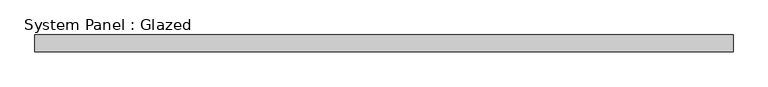
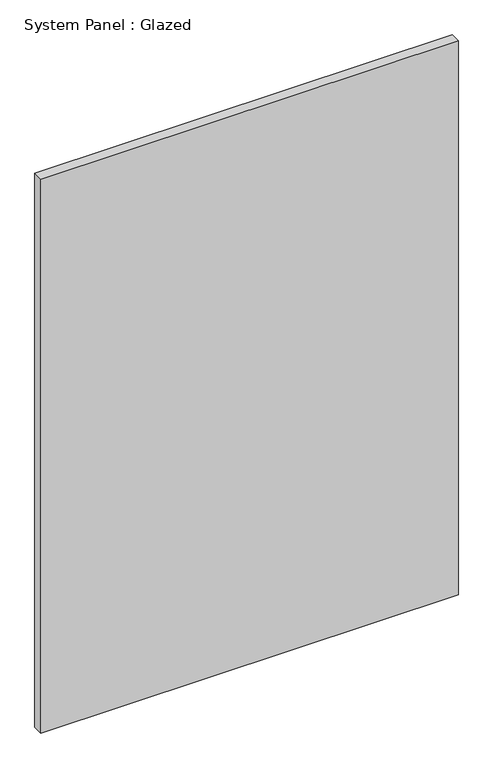
"""IFC4 building model written with IfcOpenShell, lengths in millimetres: plate geometry, System Panel : Glazed."""

from ifc_helpers import new_model, si_unit, origin, origin_with_axes, place, context, project, spatial, polyline, outline, extrude, source, transform, mapped, element, save


def system_panel_glazed_645b7f4f(model_context):
    return source(origin(), model_context, "Body", "SweptSolid", [
        extrude(outline(polyline([(526.2186578, 19.05), (-526.2186578, 19.05), (-526.2186578, 44.45), (526.2186578, 44.45), (526.2186578, 19.05)])), origin_with_axes(), (0.0, 0.0, 1.0), 1475.5825326),
    ])


if __name__ == "__main__":
    model = new_model("IFC4")
    model_context = context("Model", 3, world=origin())
    ifc_project = project(units=[si_unit("LENGTHUNIT", "METRE", prefix="MILLI")], contexts=[model_context])
    site = spatial("IfcSite", under=ifc_project)
    building = spatial("IfcBuilding", under=site)
    placement = place(None, origin())
    system_panel_glazed_shape = system_panel_glazed_645b7f4f(model_context)
    element("IfcPlate", 1, ObjectType="System Panel : Glazed", at=placement, inside=building, context=model_context, shape_type="MappedRepresentation", body=[
        mapped(system_panel_glazed_shape, transform((0.0, 0.0, 0.0), x_axis=(1.0, 0.0, 0.0), y_axis=(0.0, 1.0, 0.0), z_axis=(0.0, 0.0, 1.0))),
    ])
    save(model, "model.ifc")

# Revit data of these elements
# Type "System Panel : Glazed"
#   Construction Type Id = "GSP4R"
#   Analytic Construction = "1/8 in Pilkington single glazing"
#   Visual Light Transmittance = 0.9
#   Solar Heat Gain Coefficient = 0.86
#   Heat Transfer Coefficient (U) = 1.18115 BTU/(h·ft²·°F)
#   Define Thermal Properties by = 1
# Element 1 (IfcPlate, "System Panel : Glazed")
#   Materials on its faces: "Glass"
# Materials
#   "Glass": class "Glass", colour RGB 0 128 192, transparency 0.75, Description = "Soda Lime Glass", Cost = 0
